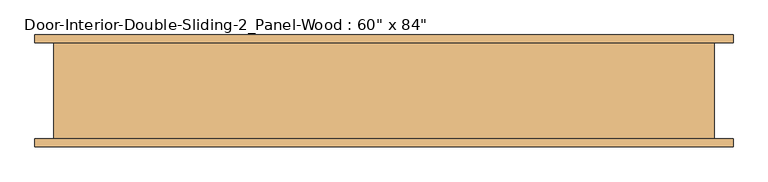
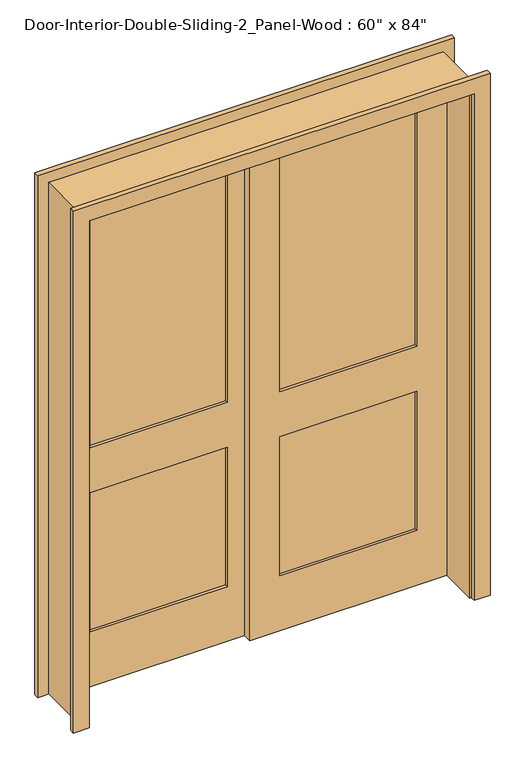
"""IFC4 building model written with IfcOpenShell, lengths in millimetres: door geometry."""

from ifc_helpers import new_model, si_unit, frame, origin, place, context, project, spatial, polyline, outline, extrude, source, transform, mapped, element, save


def door_f5864cb8(model_context):
    return source(origin(), model_context, "Body", "SweptSolid", [
        extrude(outline(polyline([(641.35, 52.9166667), (95.25, 52.9166667), (95.25, 64.5583333), (641.35, 64.5583333), (641.35, 52.9166667)])), frame((0.0, 0.0, 1009.65), z_axis=(0.0, 0.0, 1.0), x_axis=(1.0, 0.0, 0.0)), (0.0, 0.0, 1.0), 1004.8875),
        extrude(outline(polyline([(641.35, 52.9166667), (95.25, 52.9166667), (95.25, 64.5583333), (641.35, 64.5583333), (641.35, 52.9166667)])), frame((0.0, 0.0, 231.775), z_axis=(0.0, 0.0, 1.0), x_axis=(1.0, 0.0, 0.0)), (0.0, 0.0, 1.0), 587.375),
        extrude(outline(polyline([(2133.6, -25.4), (0.0, -25.4), (0.0, 762.0), (2133.6, 762.0), (2133.6, -25.4)]), holes=[polyline([(2014.5375, 95.25), (2014.5375, 641.35), (1009.65, 641.35), (1009.65, 95.25), (2014.5375, 95.25)]), polyline([(819.15, 95.25), (819.15, 641.35), (231.775, 641.35), (231.775, 95.25), (819.15, 95.25)])]), frame((0.0, 41.275, 0.0), z_axis=(0.0, 1.0, 0.0), x_axis=(0.0, 0.0, 1.0)), (0.0, 0.0, 1.0), 34.925),
        extrude(outline(polyline([(-95.25, 87.8416667), (-641.35, 87.8416667), (-641.35, 99.4833333), (-95.25, 99.4833333), (-95.25, 87.8416667)])), frame((0.0, 0.0, 1009.65), z_axis=(0.0, 0.0, 1.0), x_axis=(1.0, 0.0, 0.0)), (0.0, 0.0, 1.0), 1004.8875),
        extrude(outline(polyline([(-95.25, 87.8416667), (-641.35, 87.8416667), (-641.35, 99.4833333), (-95.25, 99.4833333), (-95.25, 87.8416667)])), frame((0.0, 0.0, 231.775), z_axis=(0.0, 0.0, 1.0), x_axis=(1.0, 0.0, 0.0)), (0.0, 0.0, 1.0), 587.375),
        extrude(outline(polyline([(2133.6, -762.0), (0.0, -762.0), (0.0, 25.4), (2133.6, 25.4), (2133.6, -762.0)]), holes=[polyline([(2014.5375, -641.35), (2014.5375, -95.25), (1009.65, -95.25), (1009.65, -641.35), (2014.5375, -641.35)]), polyline([(819.15, -641.35), (819.15, -95.25), (231.775, -95.25), (231.775, -641.35), (819.15, -641.35)])]), frame((0.0, 76.2, 0.0), z_axis=(0.0, 1.0, 0.0), x_axis=(0.0, 0.0, 1.0)), (0.0, 0.0, 1.0), 34.925),
        extrude(outline(polyline([(0.0, 762.0), (0.0, 787.4), (2159.0, 787.4), (2159.0, -787.4), (0.0, -787.4), (0.0, -762.0), (2133.6, -762.0), (2133.6, 762.0), (0.0, 762.0)])), frame((0.0, -117.475, 0.0), z_axis=(0.0, 1.0, 0.0), x_axis=(0.0, 0.0, 1.0)), (0.0, 0.0, 1.0), 228.6),
        extrude(outline(polyline([(0.0, 768.35), (0.0, 831.85), (2203.45, 831.85), (2203.45, -831.85), (0.0, -831.85), (0.0, -768.35), (2139.95, -768.35), (2139.95, 768.35), (0.0, 768.35)])), frame((0.0, -136.525, 0.0), z_axis=(0.0, 1.0, 0.0), x_axis=(0.0, 0.0, 1.0)), (0.0, 0.0, 1.0), 19.05),
        extrude(outline(polyline([(0.0, 768.35), (0.0, 831.85), (2203.45, 831.85), (2203.45, -831.85), (0.0, -831.85), (0.0, -768.35), (2139.95, -768.35), (2139.95, 768.35), (0.0, 768.35)])), frame((0.0, 111.125, 0.0), z_axis=(0.0, 1.0, 0.0), x_axis=(0.0, 0.0, 1.0)), (0.0, 0.0, 1.0), 19.05),
    ])


if __name__ == "__main__":
    model = new_model("IFC4")
    model_context = context("Model", 3, world=origin())
    ifc_project = project(units=[si_unit("LENGTHUNIT", "METRE", prefix="MILLI")], contexts=[model_context])
    site = spatial("IfcSite", under=ifc_project)
    building = spatial("IfcBuilding", under=site)
    placement = place(None, origin())
    door_shape = door_f5864cb8(model_context)
    element("IfcDoor", 1, ObjectType="Door-Interior-Double-Sliding-2_Panel-Wood : 60\" x 84\"", at=placement, inside=building, context=model_context, shape_type="MappedRepresentation", body=[
        mapped(door_shape, transform((0.0, 0.0, 0.0), x_axis=(1.0, 0.0, 0.0), y_axis=(0.0, 1.0, 0.0), z_axis=(0.0, 0.0, 1.0))),
    ])
    save(model, "model.ifc")

# Revit data of these elements
# Type "Door-Interior-Double-Sliding-2_Panel-Wood : 60\" x 84\""
#   Type Mark = "8"
#   Assembly Code = "C1020300"
#   Analytic Construction = "Wooden"
#   Top Rail = 0' - 4 11/16"
#   Thickness = 0' - 1 3/8"
#   Thermal Resistance (R) = 2.5876 (h·ft²·°F)/BTU
#   Stiles = 0' - 4 3/4"
#   Rough Width = 5' - 2"
#   Rough Height = 7' - 1"
#   Lock Rail = 0' - 7 1/2"
#   Height = 7' - 0"
#   Width = 5' - 0"
#   Heat Transfer Coefficient (U) = 0.3865 BTU/(h·ft²·°F)
#   Bottom Rail = 0' - 9 1/8"
#   Trim Material = Cherry
#   Panel Material = Cherry
#   Frame Material = Cherry
#   Visual Light Transmittance = 0
#   Solar Heat Gain Coefficient = 0
#   Wall Closure = (empty or 0)
#   Function = (empty or 0)
# Element 1 (IfcDoor, "Door-Interior-Double-Sliding-2_Panel-Wood : 60\" x 84\"")
#   Materials on its faces: "Cherry"
# Materials
#   "Cherry": class "Wood", colour RGB 226 177 128, transparency 0, Description = "Prunus Serotina", Cost = 0
